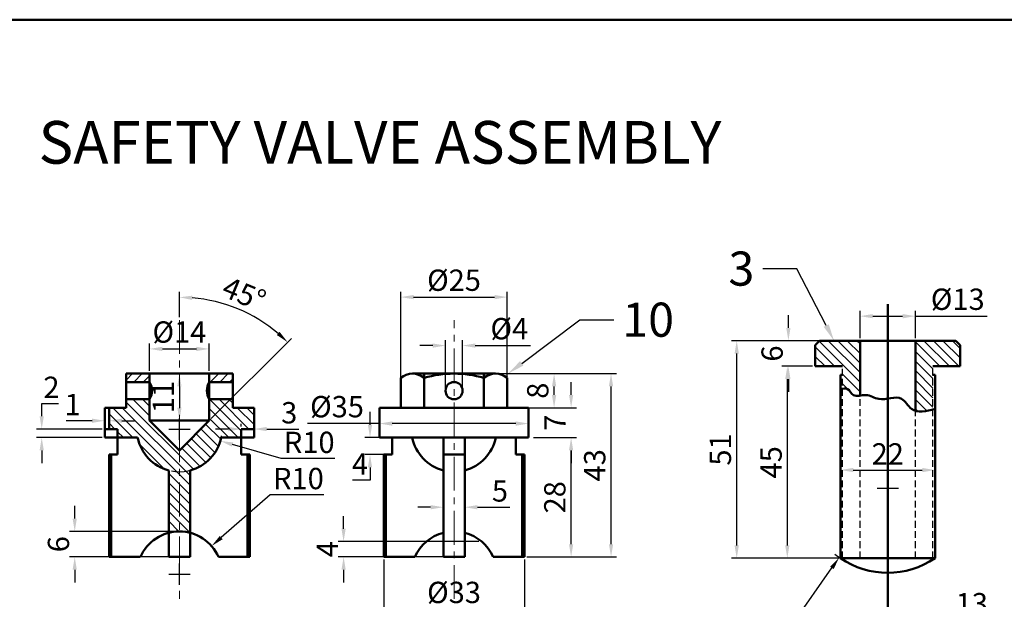
# Model space of a CAD drawing. Units: millimetres. Extents: x -656 to 85, y 134 to 571.
# Tile 4 of 5: x -409 to -178, y 435 to 571. Entities that reach past the tile are written whole.
import ezdxf
from ezdxf import colors
from ezdxf.entities.mleader import LeaderData, LeaderLine
from ezdxf.math import Vec2, Vec3

# ---------------------------------------------------------------- set-up
doc = ezdxf.new("R2010")
doc.units = ezdxf.units.MM
doc.header["$LTSCALE"] = 0.5
doc.linetypes.add('CENTER', pattern=[50.8, 31.75, -6.35, 6.35, -6.35])
doc.linetypes.add('HIDDEN', pattern=[9.525, 6.35, -3.175])
for name, color, linetype, lineweight in [('M-CNTR', 1, 'CENTER', 18), ('M-DIMS', 2, 'Continuous', 25), ('M-HATC', 8, 'Continuous', 18), ('M-HIDN', 3, 'HIDDEN', 25), ('M-OUTL', 7, 'Continuous', 50), ('M-TEXT', 7, 'Continuous', 25), ('M-TTLB', 7, 'Continuous', 50)]:
    doc.layers.add(name, color=color, linetype=linetype, lineweight=lineweight)
doc.styles.get("Standard").update_dxf_attribs({"font": 'arial.ttf'})
doc.dimstyles.new('ISO-25', dxfattribs={"dimtxt": 5, "dimasz": 3, "dimexe": 1.25, "dimexo": 0.625, "dimtad": 1, "dimtoh": 1, "dimdec": 0, "dimtxsty": 'Standard', "dimcen": 2.5, "dimadec": 0, "dimazin": 0, "dimtfac": 1, "dimtdec": 0, "dimtofl": 0, "dimtmove": 0, "dimatfit": 3, "dimfxl": 1, "dimarcsym": 0})

# ---------------------------------------------------------------- blocks, each defined once
blk = doc.blocks.new('*D33')
at = {"layer": 'Defpoints', "color": 0, "ltscale": 0.5, "transparency": 16777216}
for p in [(-323.49, 445.02), (-290.49, 445.02), (-290.49, 432.74)]:
    blk.add_point(p, dxfattribs=at)
at = {"layer": 'M-DIMS', "color": 0, "lineweight": -2, "ltscale": 0.5, "transparency": 16777216}
for p, q in [((-323.49, 444.4), (-323.49, 431.49)), ((-290.49, 444.4), (-290.49, 431.49)), ((-320.49, 432.74), (-293.49, 432.74))]:
    blk.add_line(p, q, dxfattribs=at)
at = {"layer": 'M-DIMS', "color": 0, "ltscale": 0.5, "transparency": 16777216}
for points in [[(-320.49, 433.24), (-320.49, 432.24), (-323.49, 432.74)], [(-293.49, 433.24), (-293.49, 432.24), (-290.49, 432.74)]]:
    blk.add_solid(points, dxfattribs=at)
at = {"layer": 'M-DIMS', "color": 0, "ltscale": 0.5, "transparency": 16777216, "insert": (-306.99, 436.06), "char_height": 5, "attachment_point": 5}
blk.add_mtext('%%C33', dxfattribs=at)
blk = doc.blocks.new('*D34')
at = {"layer": 'Defpoints', "color": 0, "ltscale": 0.5, "transparency": 16777216}
for p in [(-304.49, 456.69), (-309.49, 448.8), (-304.49, 448.8)]:
    blk.add_point(p, dxfattribs=at)
at = {"layer": 'M-DIMS', "color": 0, "lineweight": -2, "ltscale": 0.5, "transparency": 16777216}
for p, q in [((-309.49, 449.42), (-309.49, 457.94)), ((-304.49, 449.42), (-304.49, 457.94)), ((-312.49, 456.69), (-315.49, 456.69)), ((-301.49, 456.69), (-293.93, 456.69))]:
    blk.add_line(p, q, dxfattribs=at)
at = {"layer": 'M-DIMS', "color": 0, "ltscale": 0.5, "transparency": 16777216}
for points in [[(-312.49, 457.19), (-312.49, 456.19), (-309.49, 456.69)], [(-301.49, 457.19), (-301.49, 456.19), (-304.49, 456.69)]]:
    blk.add_solid(points, dxfattribs=at)
at = {"layer": 'M-DIMS', "color": 0, "ltscale": 0.5, "transparency": 16777216, "insert": (-296.21, 459.86), "char_height": 5, "attachment_point": 5}
blk.add_mtext('5', dxfattribs=at)
blk = doc.blocks.new('*D35')
at = {"layer": 'Defpoints', "color": 0, "ltscale": 0.5, "transparency": 16777216}
for p in [(-288.99, 473.02), (-279.52, 473.02), (-290.49, 445.02)]:
    blk.add_point(p, dxfattribs=at)
at = {"layer": 'M-DIMS', "color": 0, "lineweight": -2, "ltscale": 0.5, "transparency": 16777216}
for p, q in [((-288.37, 473.02), (-278.27, 473.02)), ((-279.52, 448.02), (-279.52, 470.02)), ((-289.87, 445.02), (-278.27, 445.02))]:
    blk.add_line(p, q, dxfattribs=at)
at = {"layer": 'M-DIMS', "color": 0, "ltscale": 0.5, "transparency": 16777216}
for points in [[(-280.02, 470.02), (-279.02, 470.02), (-279.52, 473.02)], [(-280.02, 448.02), (-279.02, 448.02), (-279.52, 445.02)]]:
    blk.add_solid(points, dxfattribs=at)
at = {"layer": 'M-DIMS', "color": 0, "ltscale": 0.5, "transparency": 16777216, "insert": (-282.69, 459.02), "char_height": 5, "attachment_point": 5, "rotation": 90}
blk.add_mtext('28', dxfattribs=at)
blk = doc.blocks.new('*D36')
at = {"layer": 'Defpoints', "color": 0, "ltscale": 0.5, "transparency": 16777216}
for p in [(-288.99, 480.02), (-279.52, 480.02), (-288.99, 473.02)]:
    blk.add_point(p, dxfattribs=at)
at = {"layer": 'M-DIMS', "color": 0, "lineweight": -2, "ltscale": 0.5, "transparency": 16777216}
for p, q in [((-279.52, 483.02), (-279.52, 486.02)), ((-288.37, 480.02), (-278.27, 480.02)), ((-288.37, 473.02), (-278.27, 473.02)), ((-279.52, 470.02), (-279.52, 467.02))]:
    blk.add_line(p, q, dxfattribs=at)
at = {"layer": 'M-DIMS', "color": 0, "ltscale": 0.5, "transparency": 16777216}
for points in [[(-280.02, 483.02), (-279.02, 483.02), (-279.52, 480.02)], [(-280.02, 470.02), (-279.02, 470.02), (-279.52, 473.02)]]:
    blk.add_solid(points, dxfattribs=at)
at = {"layer": 'M-DIMS', "color": 0, "ltscale": 0.5, "transparency": 16777216, "insert": (-282.64, 476.52), "char_height": 5, "attachment_point": 5, "rotation": 90}
blk.add_mtext('7', dxfattribs=at)
blk = doc.blocks.new('*D37')
at = {"layer": 'Defpoints', "color": 0, "ltscale": 0.5, "transparency": 16777216}
for p in [(-306.99, 488.02), (-270.15, 488.02), (-290.49, 445.02)]:
    blk.add_point(p, dxfattribs=at)
at = {"layer": 'M-DIMS', "color": 0, "lineweight": -2, "ltscale": 0.5, "transparency": 16777216}
for p, q in [((-306.37, 488.02), (-268.9, 488.02)), ((-270.15, 448.02), (-270.15, 485.02)), ((-289.87, 445.02), (-268.9, 445.02))]:
    blk.add_line(p, q, dxfattribs=at)
at = {"layer": 'M-DIMS', "color": 0, "ltscale": 0.5, "transparency": 16777216}
for points in [[(-270.65, 485.02), (-269.65, 485.02), (-270.15, 488.02)], [(-270.65, 448.02), (-269.65, 448.02), (-270.15, 445.02)]]:
    blk.add_solid(points, dxfattribs=at)
at = {"layer": 'M-DIMS', "color": 0, "ltscale": 0.5, "transparency": 16777216, "insert": (-273.33, 466.52), "char_height": 5, "attachment_point": 5, "rotation": 90}
blk.add_mtext('43', dxfattribs=at)
blk = doc.blocks.new('*D38')
at = {"layer": 'Defpoints', "color": 0, "ltscale": 0.5, "transparency": 16777216}
for p in [(-306.99, 488.02), (-283.51, 488.02), (-294.49, 480.02)]:
    blk.add_point(p, dxfattribs=at)
at = {"layer": 'M-DIMS', "color": 0, "lineweight": -2, "ltscale": 0.5, "transparency": 16777216}
for p, q in [((-306.37, 488.02), (-282.26, 488.02)), ((-283.51, 483.02), (-283.51, 485.02)), ((-293.87, 480.02), (-282.26, 480.02))]:
    blk.add_line(p, q, dxfattribs=at)
at = {"layer": 'M-DIMS', "color": 0, "ltscale": 0.5, "transparency": 16777216}
for points in [[(-284.01, 485.02), (-283.01, 485.02), (-283.51, 488.02)], [(-284.01, 483.02), (-283.01, 483.02), (-283.51, 480.02)]]:
    blk.add_solid(points, dxfattribs=at)
at = {"layer": 'M-DIMS', "color": 0, "ltscale": 0.5, "transparency": 16777216, "insert": (-286.69, 484.02), "char_height": 5, "attachment_point": 5, "rotation": 90}
blk.add_mtext('8', dxfattribs=at)
blk = doc.blocks.new('*D39')
at = {"layer": 'Defpoints', "color": 0, "ltscale": 0.5, "transparency": 16777216}
for p in [(-294.49, 505.96), (-319.49, 483.52), (-294.49, 483.52)]:
    blk.add_point(p, dxfattribs=at)
at = {"layer": 'M-DIMS', "color": 0, "lineweight": -2, "ltscale": 0.5, "transparency": 16777216}
for p, q in [((-319.49, 484.15), (-319.49, 507.21)), ((-316.49, 505.96), (-297.49, 505.96)), ((-294.49, 484.15), (-294.49, 507.21))]:
    blk.add_line(p, q, dxfattribs=at)
at = {"layer": 'M-DIMS', "color": 0, "ltscale": 0.5, "transparency": 16777216}
for points in [[(-316.49, 506.46), (-316.49, 505.46), (-319.49, 505.96)], [(-297.49, 506.46), (-297.49, 505.46), (-294.49, 505.96)]]:
    blk.add_solid(points, dxfattribs=at)
at = {"layer": 'M-DIMS', "color": 0, "ltscale": 0.5, "transparency": 16777216, "insert": (-306.99, 509.28), "char_height": 5, "attachment_point": 5}
blk.add_mtext('%%C25', dxfattribs=at)
blk = doc.blocks.new('*D40')
at = {"layer": 'Defpoints', "color": 0, "ltscale": 0.5, "transparency": 16777216}
for p in [(-304.99, 494.59), (-308.99, 484.02), (-304.99, 484.02)]:
    blk.add_point(p, dxfattribs=at)
at = {"layer": 'M-DIMS', "color": 0, "lineweight": -2, "ltscale": 0.5, "transparency": 16777216}
for p, q in [((-311.99, 494.59), (-314.99, 494.59)), ((-308.99, 484.65), (-308.99, 495.84)), ((-304.99, 484.65), (-304.99, 495.84)), ((-301.99, 494.59), (-289.04, 494.59))]:
    blk.add_line(p, q, dxfattribs=at)
at = {"layer": 'M-DIMS', "color": 0, "ltscale": 0.5, "transparency": 16777216}
for points in [[(-311.99, 495.09), (-311.99, 494.09), (-308.99, 494.59)], [(-301.99, 495.09), (-301.99, 494.09), (-304.99, 494.59)]]:
    blk.add_solid(points, dxfattribs=at)
at = {"layer": 'M-DIMS', "color": 0, "ltscale": 0.5, "transparency": 16777216, "insert": (-294.02, 497.91), "char_height": 5, "attachment_point": 5}
blk.add_mtext('%%C4', dxfattribs=at)
blk = doc.blocks.new('*D41')
at = {"layer": 'Defpoints', "color": 0, "ltscale": 0.5, "transparency": 16777216}
for p in [(-324.49, 476.52), (-289.49, 476.52), (-289.49, 476.31)]:
    blk.add_point(p, dxfattribs=at)
at = {"layer": 'M-DIMS', "color": 0, "lineweight": -2, "ltscale": 0.5, "transparency": 16777216}
for p, q in [((-324.49, 476.31), (-341.38, 476.31)), ((-292.49, 476.31), (-321.49, 476.31)), ((-324.49, 475.9), (-324.49, 475.06)), ((-289.49, 475.9), (-289.49, 475.06))]:
    blk.add_line(p, q, dxfattribs=at)
at = {"layer": 'M-DIMS', "color": 0, "ltscale": 0.5, "transparency": 16777216}
for points in [[(-321.49, 476.81), (-321.49, 475.81), (-324.49, 476.31)], [(-292.49, 476.81), (-292.49, 475.81), (-289.49, 476.31)]]:
    blk.add_solid(points, dxfattribs=at)
at = {"layer": 'M-DIMS', "color": 0, "ltscale": 0.5, "transparency": 16777216, "insert": (-334.44, 479.62), "char_height": 5, "attachment_point": 5}
blk.add_mtext('%%C35', dxfattribs=at)
blk = doc.blocks.new('*D42')
at = {"layer": 'Defpoints', "color": 0, "ltscale": 0.5, "transparency": 16777216}
for p in [(-321.49, 473.02), (-326.7, 469.02), (-321.49, 469.02)]:
    blk.add_point(p, dxfattribs=at)
at = {"layer": 'M-DIMS', "color": 0, "lineweight": -2, "ltscale": 0.5, "transparency": 16777216}
for p, q in [((-326.7, 476.02), (-326.7, 479.02)), ((-322.12, 473.02), (-327.95, 473.02)), ((-322.12, 469.02), (-327.95, 469.02)), ((-326.7, 466.02), (-326.7, 463.02)), ((-326.7, 463.02), (-330.78, 463.02))]:
    blk.add_line(p, q, dxfattribs=at)
at = {"layer": 'M-DIMS', "color": 0, "ltscale": 0.5, "transparency": 16777216}
for points in [[(-327.2, 476.02), (-326.2, 476.02), (-326.7, 473.02)], [(-327.2, 466.02), (-326.2, 466.02), (-326.7, 469.02)]]:
    blk.add_solid(points, dxfattribs=at)
at = {"layer": 'M-DIMS', "color": 0, "ltscale": 0.5, "transparency": 16777216, "insert": (-329.05, 466.15), "char_height": 5, "attachment_point": 5}
blk.add_mtext('4', dxfattribs=at)
blk = doc.blocks.new('*D43')
at = {"layer": 'Defpoints', "color": 0, "ltscale": 0.5, "transparency": 16777216}
for p in [(-364.42, 493.81), (-378.42, 488.02), (-364.42, 488.02)]:
    blk.add_point(p, dxfattribs=at)
at = {"layer": 'M-DIMS', "color": 0, "lineweight": -2, "ltscale": 0.5, "transparency": 16777216}
for p, q in [((-378.42, 488.65), (-378.42, 495.06)), ((-364.42, 488.65), (-364.42, 495.06)), ((-375.42, 493.81), (-367.42, 493.81))]:
    blk.add_line(p, q, dxfattribs=at)
at = {"layer": 'M-DIMS', "color": 0, "ltscale": 0.5, "transparency": 16777216}
for points in [[(-375.42, 494.31), (-375.42, 493.31), (-378.42, 493.81)], [(-367.42, 494.31), (-367.42, 493.31), (-364.42, 493.81)]]:
    blk.add_solid(points, dxfattribs=at)
at = {"layer": 'M-DIMS', "color": 0, "ltscale": 0.5, "transparency": 16777216, "insert": (-371.42, 497.12), "char_height": 5, "attachment_point": 5}
blk.add_mtext('%%C14', dxfattribs=at)
blk = doc.blocks.new('*D44')
at = {"layer": 'Defpoints', "color": 0, "ltscale": 0.5, "transparency": 16777216}
for p in [(-403.73, 475.02), (-388.92, 475.02), (-388.92, 473.02)]:
    blk.add_point(p, dxfattribs=at)
at = {"layer": 'M-DIMS', "color": 0, "lineweight": -2, "ltscale": 0.5, "transparency": 16777216}
for p, q in [((-403.73, 478.02), (-403.73, 481.02)), ((-403.73, 481.02), (-399.79, 481.02)), ((-389.55, 475.02), (-404.98, 475.02)), ((-389.55, 473.02), (-404.98, 473.02)), ((-403.73, 470.02), (-403.73, 467.02))]:
    blk.add_line(p, q, dxfattribs=at)
at = {"layer": 'M-DIMS', "color": 0, "ltscale": 0.5, "transparency": 16777216}
for points in [[(-404.23, 478.02), (-403.23, 478.02), (-403.73, 475.02)], [(-404.23, 470.02), (-403.23, 470.02), (-403.73, 473.02)]]:
    blk.add_solid(points, dxfattribs=at)
at = {"layer": 'M-DIMS', "color": 0, "ltscale": 0.5, "transparency": 16777216, "insert": (-401.44, 484.16), "char_height": 5, "attachment_point": 5}
blk.add_mtext('2', dxfattribs=at)
blk = doc.blocks.new('*D45')
at = {"layer": 'Defpoints', "color": 0, "ltscale": 0.5, "transparency": 16777216}
for p in [(-388.92, 476.52), (-387.92, 476.97), (-387.92, 476.52)]:
    blk.add_point(p, dxfattribs=at)
at = {"layer": 'M-DIMS', "color": 0, "lineweight": -2, "ltscale": 0.5, "transparency": 16777216}
for p, q in [((-388.92, 477.15), (-388.92, 478.22)), ((-387.92, 477.15), (-387.92, 478.22)), ((-391.92, 476.97), (-398.01, 476.97)), ((-384.92, 476.97), (-381.92, 476.97))]:
    blk.add_line(p, q, dxfattribs=at)
at = {"layer": 'M-DIMS', "color": 0, "ltscale": 0.5, "transparency": 16777216}
for points in [[(-391.92, 477.47), (-391.92, 476.47), (-388.92, 476.97)], [(-384.92, 477.47), (-384.92, 476.47), (-387.92, 476.97)]]:
    blk.add_solid(points, dxfattribs=at)
at = {"layer": 'M-DIMS', "color": 0, "ltscale": 0.5, "transparency": 16777216, "insert": (-396.47, 480.11), "char_height": 5, "attachment_point": 5}
blk.add_mtext('1', dxfattribs=at)
blk = doc.blocks.new('*D46')
at = {"layer": 'Defpoints', "color": 0, "ltscale": 0.5, "transparency": 16777216}
for p in [(-356.92, 475.02), (-353.92, 475.02), (-353.92, 475.02)]:
    blk.add_point(p, dxfattribs=at)
at = {"layer": 'M-DIMS', "color": 0, "lineweight": -2, "ltscale": 0.5, "transparency": 16777216}
for p, q in [((-356.92, 475.65), (-356.92, 476.27)), ((-353.92, 475.65), (-353.92, 476.27)), ((-359.92, 475.02), (-362.92, 475.02)), ((-350.92, 475.02), (-343.4, 475.02))]:
    blk.add_line(p, q, dxfattribs=at)
at = {"layer": 'M-DIMS', "color": 0, "ltscale": 0.5, "transparency": 16777216}
for points in [[(-359.92, 475.52), (-359.92, 474.52), (-356.92, 475.02)], [(-350.92, 475.52), (-350.92, 474.52), (-353.92, 475.02)]]:
    blk.add_solid(points, dxfattribs=at)
at = {"layer": 'M-DIMS', "color": 0, "ltscale": 0.5, "transparency": 16777216, "insert": (-345.66, 478.2), "char_height": 5, "attachment_point": 5}
blk.add_mtext('3', dxfattribs=at)
blk = doc.blocks.new('*D47')
at = {"layer": 'Defpoints', "color": 0, "ltscale": 0.5, "transparency": 16777216}
for p in [(-371.42, 475.02), (-361.82, 472.23)]:
    blk.add_point(p, dxfattribs=at)
at = {"layer": 'M-DIMS', "color": 0, "lineweight": -2, "ltscale": 0.5, "transparency": 16777216}
for p, q in [((-371.42, 472.52), (-371.42, 477.52)), ((-373.92, 475.02), (-368.92, 475.02)), ((-347.55, 468.08), (-358.94, 471.39)), ((-334.99, 468.08), (-347.55, 468.08))]:
    blk.add_line(p, q, dxfattribs=at)
blk.add_arc((-371.42, 475.02), 10, 259.1035, 350.9346, dxfattribs=at)
at = {"layer": 'M-DIMS', "color": 0, "ltscale": 0.5, "transparency": 16777216}
blk.add_solid([(-358.8, 471.87), (-359.08, 470.91), (-361.82, 472.23)], dxfattribs=at)
at = {"layer": 'M-DIMS', "color": 0, "ltscale": 0.5, "transparency": 16777216, "insert": (-340.96, 471.25), "char_height": 5, "attachment_point": 5}
blk.add_mtext('R10', dxfattribs=at)
blk = doc.blocks.new('*D48')
at = {"layer": 'Defpoints', "color": 0, "ltscale": 0.5, "transparency": 16777216}
for p in [(-371.42, 500.59), (-353.47, 501.11), (-364.42, 477.02), (-371.42, 470.02), (-371.42, 435.19)]:
    blk.add_point(p, dxfattribs=at)
at = {"layer": 'M-DIMS', "color": 0, "lineweight": -2, "ltscale": 0.5, "transparency": 16777216}
for p, q in [((-371.42, 501.22), (-371.42, 507.17)), ((-363.98, 477.47), (-345.15, 496.29))]:
    blk.add_line(p, q, dxfattribs=at)
blk.add_arc((-371.42, 470.02), 35.9, 49.7896, 85.2104, dxfattribs=at)
at = {"layer": 'M-DIMS', "color": 0, "ltscale": 0.5, "transparency": 16777216}
for points in [[(-368.45, 505.3), (-368.4, 506.3), (-371.42, 505.92)], [(-347.91, 497.81), (-348.58, 497.07), (-346.04, 495.41)]]:
    blk.add_solid(points, dxfattribs=at)
at = {"layer": 'M-DIMS', "color": 0, "ltscale": 0.5, "transparency": 16777216, "insert": (-356.47, 506.12), "char_height": 5, "attachment_point": 5, "rotation": 337.5}
blk.add_mtext('45°', dxfattribs=at)
blk = doc.blocks.new('*D49')
at = {"layer": 'Defpoints', "color": 0, "ltscale": 0.5, "transparency": 16777216}
for p in [(-372.99, 488.02), (-372.99, 477.02), (-371.42, 477.02)]:
    blk.add_point(p, dxfattribs=at)
at = {"layer": 'M-DIMS', "color": 0, "lineweight": -2, "ltscale": 0.5, "transparency": 16777216}
for p, q in [((-372.36, 488.02), (-370.17, 488.02)), ((-371.42, 485.02), (-371.42, 480.02)), ((-372.36, 477.02), (-370.17, 477.02))]:
    blk.add_line(p, q, dxfattribs=at)
at = {"layer": 'M-DIMS', "color": 0, "ltscale": 0.5, "transparency": 16777216}
for points in [[(-371.92, 485.02), (-370.92, 485.02), (-371.42, 488.02)], [(-371.92, 480.02), (-370.92, 480.02), (-371.42, 477.02)]]:
    blk.add_solid(points, dxfattribs=at)
at = {"layer": 'M-DIMS', "color": 0, "ltscale": 0.5, "transparency": 16777216, "insert": (-374.56, 482.52), "char_height": 5, "attachment_point": 5, "rotation": 90}
blk.add_mtext('11', dxfattribs=at)
blk = doc.blocks.new('*D51')
at = {"layer": 'Defpoints', "color": 0, "ltscale": 0.5, "transparency": 16777216}
for p in [(-200.1, 422), (-200.08, 421.98), (-210.36, 414.02)]:
    blk.add_point(p, dxfattribs=at)
at = {"layer": 'M-DIMS', "color": 0, "lineweight": -2, "ltscale": 0.5, "transparency": 16777216}
for p, q in [((-200.08, 421.98), (-189.47, 430.24)), ((-189.47, 430.24), (-182.15, 430.24)), ((-199.72, 421.51), (-199.32, 420.99)), ((-207.97, 415.83), (-202.45, 420.13)), ((-209.98, 413.52), (-209.57, 413.01))]:
    blk.add_line(p, q, dxfattribs=at)
at = {"layer": 'M-DIMS', "color": 0, "ltscale": 0.5, "transparency": 16777216}
for points in [[(-202.76, 420.53), (-202.14, 419.74), (-200.08, 421.98)], [(-208.28, 416.23), (-207.67, 415.44), (-210.34, 413.99)]]:
    blk.add_solid(points, dxfattribs=at)
at = {"layer": 'M-DIMS', "color": 0, "ltscale": 0.5, "transparency": 16777216, "insert": (-185.5, 433.42), "char_height": 5, "attachment_point": 5}
blk.add_mtext('13', dxfattribs=at)
blk = doc.blocks.new('*D52')
at = {"layer": 'Defpoints', "color": 0, "ltscale": 0.5, "transparency": 16777216}
for p in [(-228.54, 495.73), (-205.23, 495.73), (-222.23, 489.73)]:
    blk.add_point(p, dxfattribs=at)
at = {"layer": 'M-DIMS', "color": 0, "lineweight": -2, "ltscale": 0.5, "transparency": 16777216}
for p, q in [((-228.54, 498.73), (-228.54, 501.73)), ((-205.86, 495.73), (-229.79, 495.73)), ((-222.86, 489.73), (-229.79, 489.73)), ((-228.54, 486.73), (-228.54, 483.73))]:
    blk.add_line(p, q, dxfattribs=at)
at = {"layer": 'M-DIMS', "color": 0, "ltscale": 0.5, "transparency": 16777216}
for points in [[(-229.04, 498.73), (-228.04, 498.73), (-228.54, 495.73)], [(-229.04, 486.73), (-228.04, 486.73), (-228.54, 489.73)]]:
    blk.add_solid(points, dxfattribs=at)
at = {"layer": 'M-DIMS', "color": 0, "ltscale": 0.5, "transparency": 16777216, "insert": (-231.71, 492.73), "char_height": 5, "attachment_point": 5, "rotation": 90}
blk.add_mtext('6', dxfattribs=at)
blk = doc.blocks.new('*D53')
at = {"layer": 'Defpoints', "color": 0, "ltscale": 0.5, "transparency": 16777216}
for p in [(-240.66, 495.73), (-205.23, 495.73), (-205.23, 444.73)]:
    blk.add_point(p, dxfattribs=at)
at = {"layer": 'M-DIMS', "color": 0, "lineweight": -2, "ltscale": 0.5, "transparency": 16777216}
for p, q in [((-205.86, 495.73), (-241.91, 495.73)), ((-240.66, 447.73), (-240.66, 492.73)), ((-205.86, 444.73), (-241.91, 444.73))]:
    blk.add_line(p, q, dxfattribs=at)
at = {"layer": 'M-DIMS', "color": 0, "ltscale": 0.5, "transparency": 16777216}
for points in [[(-241.16, 492.73), (-240.16, 492.73), (-240.66, 495.73)], [(-241.16, 447.73), (-240.16, 447.73), (-240.66, 444.73)]]:
    blk.add_solid(points, dxfattribs=at)
at = {"layer": 'M-DIMS', "color": 0, "ltscale": 0.5, "transparency": 16777216, "insert": (-243.84, 470.23), "char_height": 5, "attachment_point": 5, "rotation": 90}
blk.add_mtext('51', dxfattribs=at)
blk = doc.blocks.new('*D54')
at = {"layer": 'Defpoints', "color": 0, "ltscale": 0.5, "transparency": 16777216}
for p in [(-205.23, 461.18), (-216.61, 444.92)]:
    blk.add_point(p, dxfattribs=at)
at = {"layer": 'M-DIMS', "color": 0, "lineweight": -2, "ltscale": 0.5, "transparency": 16777216}
for p, q in [((-205.23, 458.68), (-205.23, 463.68)), ((-207.73, 461.18), (-202.73, 461.18)), ((-232.53, 422.16), (-218.33, 442.46)), ((-249.97, 422.16), (-232.53, 422.16))]:
    blk.add_line(p, q, dxfattribs=at)
blk.add_arc((-205.23, 461.18), 19.85, 231.4164, 235.9903, dxfattribs=at)
at = {"layer": 'M-DIMS', "color": 0, "ltscale": 0.5, "transparency": 16777216}
blk.add_solid([(-218.74, 442.75), (-217.92, 442.18), (-216.61, 444.92)], dxfattribs=at)
at = {"layer": 'M-DIMS', "color": 0, "ltscale": 0.5, "transparency": 16777216, "insert": (-244, 425.34), "char_height": 5, "attachment_point": 5}
blk.add_mtext('R20', dxfattribs=at)
blk = doc.blocks.new('*D55')
at = {"layer": 'Defpoints', "color": 0, "ltscale": 0.5, "transparency": 16777216}
for p in [(-216.33, 466.23), (-194.13, 466.23), (-194.13, 465.41)]:
    blk.add_point(p, dxfattribs=at)
at = {"layer": 'M-DIMS', "color": 0, "lineweight": -2, "ltscale": 0.5, "transparency": 16777216}
for p, q in [((-216.33, 465.61), (-216.33, 464.16)), ((-213.33, 465.41), (-197.13, 465.41)), ((-194.13, 465.61), (-194.13, 464.16))]:
    blk.add_line(p, q, dxfattribs=at)
at = {"layer": 'M-DIMS', "color": 0, "ltscale": 0.5, "transparency": 16777216}
for points in [[(-213.33, 465.91), (-213.33, 464.91), (-216.33, 465.41)], [(-197.13, 465.91), (-197.13, 464.91), (-194.13, 465.41)]]:
    blk.add_solid(points, dxfattribs=at)
at = {"layer": 'M-DIMS', "color": 0, "ltscale": 0.5, "transparency": 16777216, "insert": (-205.23, 468.54), "char_height": 5, "attachment_point": 5}
blk.add_mtext('22', dxfattribs=at)
blk = doc.blocks.new('*D71')
at = {"layer": 'Defpoints', "color": 0, "ltscale": 0.5, "transparency": 16777216}
for p in [(-222.23, 489.73), (-228.79, 444.73), (-223.88, 444.73)]:
    blk.add_point(p, dxfattribs=at)
at = {"layer": 'M-DIMS', "color": 0, "lineweight": -2, "ltscale": 0.5, "transparency": 16777216}
for p, q in [((-222.86, 489.73), (-230.04, 489.73)), ((-228.79, 486.73), (-228.79, 447.73)), ((-224.51, 444.73), (-230.04, 444.73))]:
    blk.add_line(p, q, dxfattribs=at)
at = {"layer": 'M-DIMS', "color": 0, "ltscale": 0.5, "transparency": 16777216}
for points in [[(-229.29, 486.73), (-228.29, 486.73), (-228.79, 489.73)], [(-229.29, 447.73), (-228.29, 447.73), (-228.79, 444.73)]]:
    blk.add_solid(points, dxfattribs=at)
at = {"layer": 'M-DIMS', "color": 0, "ltscale": 0.5, "transparency": 16777216, "insert": (-231.95, 467.23), "char_height": 5, "attachment_point": 5, "rotation": 90}
blk.add_mtext('45', dxfattribs=at)
blk = doc.blocks.new('*D78')
at = {"layer": 'Defpoints', "color": 0, "ltscale": 0.5, "transparency": 16777216}
for p in [(-198.73, 501.49), (-211.73, 495.73), (-198.73, 495.73)]:
    blk.add_point(p, dxfattribs=at)
at = {"layer": 'M-DIMS', "color": 0, "lineweight": -2, "ltscale": 0.5, "transparency": 16777216}
for p, q in [((-211.73, 496.36), (-211.73, 502.74)), ((-208.73, 501.49), (-201.73, 501.49)), ((-198.73, 496.36), (-198.73, 502.74)), ((-198.73, 501.49), (-181.88, 501.49))]:
    blk.add_line(p, q, dxfattribs=at)
at = {"layer": 'M-DIMS', "color": 0, "ltscale": 0.5, "transparency": 16777216}
for points in [[(-208.73, 501.99), (-208.73, 500.99), (-211.73, 501.49)], [(-201.73, 501.99), (-201.73, 500.99), (-198.73, 501.49)]]:
    blk.add_solid(points, dxfattribs=at)
at = {"layer": 'M-DIMS', "color": 0, "ltscale": 0.5, "transparency": 16777216, "insert": (-188.8, 504.81), "char_height": 5, "attachment_point": 5}
blk.add_mtext('%%C13', dxfattribs=at)
blk = doc.blocks.new('*D79')
at = {"layer": 'Defpoints', "color": 0, "ltscale": 0.5, "transparency": 16777216}
for p in [(-300.5, 448.63), (-332.9, 445.02), (-306.99, 445.02)]:
    blk.add_point(p, dxfattribs=at)
at = {"layer": 'M-DIMS', "color": 0, "lineweight": -2, "ltscale": 0.5, "transparency": 16777216}
for p, q in [((-332.9, 451.63), (-332.9, 454.63)), ((-301.13, 448.63), (-334.15, 448.63)), ((-307.62, 445.02), (-334.15, 445.02)), ((-332.9, 442.02), (-332.9, 439.02))]:
    blk.add_line(p, q, dxfattribs=at)
at = {"layer": 'M-DIMS', "color": 0, "ltscale": 0.5, "transparency": 16777216}
for points in [[(-333.4, 451.63), (-332.4, 451.63), (-332.9, 448.63)], [(-333.4, 442.02), (-332.4, 442.02), (-332.9, 445.02)]]:
    blk.add_solid(points, dxfattribs=at)
at = {"layer": 'M-DIMS', "color": 0, "ltscale": 0.5, "transparency": 16777216, "insert": (-336.03, 446.83), "char_height": 5, "attachment_point": 5, "rotation": 90}
blk.add_mtext('4', dxfattribs=at)
blk = doc.blocks.new('*D80')
at = {"layer": 'Defpoints', "color": 0, "ltscale": 0.5, "transparency": 16777216}
for p in [(-371.42, 451.02), (-395.98, 445.02), (-371.42, 445.02)]:
    blk.add_point(p, dxfattribs=at)
at = {"layer": 'M-DIMS', "color": 0, "lineweight": -2, "ltscale": 0.5, "transparency": 16777216}
for p, q in [((-395.98, 454.02), (-395.98, 457.02)), ((-372.05, 451.02), (-397.23, 451.02)), ((-372.05, 445.02), (-397.23, 445.02)), ((-395.98, 442.02), (-395.98, 439.02))]:
    blk.add_line(p, q, dxfattribs=at)
at = {"layer": 'M-DIMS', "color": 0, "ltscale": 0.5, "transparency": 16777216}
for points in [[(-396.48, 454.02), (-395.48, 454.02), (-395.98, 451.02)], [(-396.48, 442.02), (-395.48, 442.02), (-395.98, 445.02)]]:
    blk.add_solid(points, dxfattribs=at)
at = {"layer": 'M-DIMS', "color": 0, "ltscale": 0.5, "transparency": 16777216, "insert": (-399.15, 448.02), "char_height": 5, "attachment_point": 5, "rotation": 90}
blk.add_mtext('6', dxfattribs=at)
blk = doc.blocks.new('*D81')
at = {"layer": 'Defpoints', "color": 0, "ltscale": 0.5, "transparency": 16777216}
for p in [(-363.88, 447.59), (-371.42, 441.02)]:
    blk.add_point(p, dxfattribs=at)
at = {"layer": 'M-DIMS', "color": 0, "lineweight": -2, "ltscale": 0.5, "transparency": 16777216}
for p, q in [((-350.09, 459.59), (-361.62, 449.56)), ((-337.53, 459.59), (-350.09, 459.59)), ((-371.42, 438.52), (-371.42, 443.52)), ((-373.92, 441.02), (-368.92, 441.02))]:
    blk.add_line(p, q, dxfattribs=at)
at = {"layer": 'M-DIMS', "color": 0, "ltscale": 0.5, "transparency": 16777216}
blk.add_solid([(-361.95, 449.94), (-361.29, 449.18), (-363.88, 447.59)], dxfattribs=at)
at = {"layer": 'M-DIMS', "color": 0, "ltscale": 0.5, "transparency": 16777216, "insert": (-343.5, 462.77), "char_height": 5, "attachment_point": 5}
blk.add_mtext('R10', dxfattribs=at)

msp = doc.modelspace()

# ---------------------------------------------------------------- hatches: boundary and pattern name
at = {"layer": 'M-HATC', "ltscale": 0.5}
h = msp.add_hatch(dxfattribs=at)
h.set_pattern_fill('ANSI31', color=256, scale=0.5, angle=90)
h.set_pattern_definition([(135, (-1699.1516, -78.561), (-1.122532, -1.122532), [])])
edge = h.paths.add_edge_path()
edge.add_line((-211.73, 495.73), (-221.23, 495.73))
edge.add_line((-221.23, 495.73), (-222.23, 494.73))
edge.add_line((-222.23, 494.73), (-222.23, 489.73))
edge.add_line((-222.23, 489.73), (-215.83, 489.73))
edge.add_line((-215.83, 489.73), (-215.83, 484.49))
edge.add_spline(control_points=[(-215.83, 484.49), (-215.41, 484.55), (-214.33, 484.59), (-213.51, 482.67), (-212.3, 482.76), (-211.73, 482.84)], knot_values=[0.462825, 0.462825, 0.462825, 0.462825, 1.655207, 3.649135, 5.265139, 5.265139, 5.265139, 5.265139], degree=3, periodic=0)
edge.add_line((-211.73, 482.84), (-211.73, 495.73))
h.paths.add_polyline_path([(-188.23, 494.73), (-189.23, 495.73), (-198.73, 495.73), (-198.73, 489.73), (-188.23, 489.73)])
edge = h.paths.add_edge_path()
edge.add_line((-194.63, 489.73), (-198.73, 489.73))
edge.add_line((-198.73, 489.73), (-198.73, 479.3))
edge.add_spline(control_points=[(-198.73, 479.3), (-197.55, 478.95), (-196.11, 479.26), (-194.63, 479.63)], knot_values=[19.465698, 19.465698, 19.465698, 19.465698, 23.432296, 23.432296, 23.432296, 23.432296], degree=3, periodic=0)
edge.add_line((-194.63, 479.63), (-194.63, 489.73))
h = msp.add_hatch(dxfattribs=at)
h.set_pattern_fill('ANSI31', color=256, scale=0.5)
h.set_pattern_definition([(45, (-1712.0703, 33.9183), (-1.122532, 1.122532), [])])
h.paths.add_polyline_path([(-358.92, 488.02), (-364.42, 488.02), (-364.42, 486.02), (-358.92, 486.02)])
h.paths.add_polyline_path([(-378.42, 488.02), (-383.92, 488.02), (-383.92, 486.02), (-378.42, 486.02)])
edge = h.paths.add_edge_path()
edge.add_arc((-371.42, 441.02), 10, 90, 104.4775)
edge.add_line((-373.92, 450.71), (-373.92, 450.35))
edge.add_arc((-371.42, 446.02), 5, 90, 120, ccw=False)
h = msp.add_hatch(dxfattribs=at)
h.set_pattern_fill('ANSI31', color=256, scale=0.5, angle=90)
h.set_pattern_definition([(135, (-1507.2803, -236.2308), (-1.122532, -1.122532), [])])
h.paths.add_polyline_path([(-373.92, 465.34), (-373.92, 450.71, -0.063254), (-371.42, 451.02), (-371.42, 470.02), (-378.42, 477.02), (-378.42, 482.02), (-383.92, 482.02), (-383.92, 480.02), (-387.92, 480.02), (-387.92, 475.02), (-385.92, 475.02), (-385.92, 473.02), (-381.22, 473.02, 0.286677)])
h.paths.add_polyline_path([(-361.62, 473.02), (-356.92, 473.02), (-356.92, 475.02), (-353.92, 475.02), (-353.92, 480.02), (-358.92, 480.02), (-358.92, 482.02), (-364.42, 482.02), (-364.42, 477.02), (-371.42, 470.02), (-371.42, 451.02, -0.063254), (-368.92, 450.71), (-368.92, 465.34, 0.286677)])

# ---------------------------------------------------------------- linework, layer by layer
at = {"layer": 'M-CNTR', "ltscale": 0.5}
for p, q in [((-371.42, 500.59), (-371.42, 435.19)), ((-306.99, 435.19), (-306.99, 500.59))]:
    msp.add_line(p, q, dxfattribs=at)
at = {"layer": 'M-HIDN', "ltscale": 0.5}
for p, q in [((-215.83, 444.73), (-215.83, 489.73)), ((-194.63, 444.73), (-194.63, 489.73)), ((-211.73, 444.73), (-211.73, 482.84)), ((-198.73, 444.73), (-198.73, 479.3))]:
    msp.add_line(p, q, dxfattribs=at)
at = {"layer": 'M-OUTL', "ltscale": 0.5}
for p, q in [((-205.23, 394.53), (-205.23, 504.27)), ((-222.23, 494.73), (-221.23, 495.73)), ((-222.23, 489.73), (-222.23, 494.73)), ((-221.23, 495.73), (-189.23, 495.73)), ((-211.73, 482.84), (-211.73, 495.73)), ((-198.73, 479.3), (-198.73, 495.73)), ((-189.23, 495.73), (-188.23, 494.73)), ((-188.23, 494.73), (-188.23, 489.73)), ((-383.92, 480.02), (-383.92, 488.02)), ((-383.92, 488.02), (-358.92, 488.02)), ((-378.42, 477.02), (-378.42, 488.02)), ((-364.42, 488.02), (-364.42, 477.02)), ((-358.92, 488.02), (-358.92, 480.02)), ((-316.74, 488.02), (-297.24, 488.02)), ((-313.99, 480.02), (-313.99, 488.02)), ((-299.99, 488.02), (-299.99, 480.02)), ((-215.83, 489.73), (-222.23, 489.73)), ((-216.33, 444.73), (-216.33, 487.73)), ((-215.83, 487.73), (-216.33, 487.73)), ((-188.23, 489.73), (-194.63, 489.73)), ((-194.13, 487.73), (-194.63, 487.73)), ((-194.13, 444.73), (-194.13, 487.73)), ((-383.92, 486.02), (-378.42, 486.02)), ((-364.42, 486.02), (-358.92, 486.02)), ((-319.49, 480.02), (-319.49, 487.02)), ((-294.49, 487.02), (-294.49, 480.02)), ((-383.92, 482.02), (-378.42, 482.02)), ((-364.42, 482.02), (-358.92, 482.02)), ((-388.92, 473.02), (-388.92, 480.02)), ((-388.92, 480.02), (-383.92, 480.02)), ((-387.92, 475.02), (-387.92, 480.02)), ((-358.92, 480.02), (-353.92, 480.02)), ((-353.92, 480.02), (-353.92, 473.02)), ((-324.49, 473.02), (-324.49, 480.02)), ((-324.49, 480.02), (-289.49, 480.02)), ((-289.49, 480.02), (-289.49, 473.02)), ((-364.42, 477.02), (-378.42, 477.02)), ((-378.42, 477.02), (-371.42, 470.02)), ((-364.42, 477.02), (-371.42, 470.02)), ((-385.92, 475.02), (-388.92, 475.02)), ((-385.92, 475.02), (-385.92, 469.02)), ((-356.92, 475.02), (-356.92, 469.02)), ((-353.92, 475.02), (-356.92, 475.02)), ((-381.22, 473.02), (-388.92, 473.02)), ((-353.92, 473.02), (-361.62, 473.02)), ((-289.49, 473.02), (-324.49, 473.02)), ((-321.49, 473.02), (-321.49, 469.02)), ((-309.49, 473.02), (-309.49, 445.02)), ((-304.49, 473.02), (-304.49, 445.02)), ((-292.49, 473.02), (-292.49, 469.02)), ((-387.92, 469.02), (-387.92, 445.02)), ((-385.92, 469.02), (-387.92, 469.02)), ((-387.42, 469.02), (-387.42, 445.02)), ((-356.92, 469.02), (-354.92, 469.02)), ((-355.42, 469.02), (-355.42, 445.02)), ((-354.92, 469.02), (-354.92, 445.02)), ((-323.49, 469.02), (-323.49, 445.02)), ((-321.49, 469.02), (-323.49, 469.02)), ((-322.99, 469.02), (-322.99, 445.02)), ((-309.49, 469.02), (-304.49, 469.02)), ((-292.49, 469.02), (-290.49, 469.02)), ((-290.99, 469.02), (-290.99, 445.02)), ((-290.49, 469.02), (-290.49, 445.02)), ((-373.92, 465.34), (-373.92, 445.02)), ((-368.92, 465.34), (-368.92, 445.02)), ((-387.92, 445.02), (-380.59, 445.02)), ((-373.92, 445.02), (-368.92, 445.02)), ((-373.92, 445.02), (-368.92, 445.02)), ((-362.26, 445.02), (-354.92, 445.02)), ((-323.49, 445.02), (-322.99, 445.02)), ((-323.49, 445.02), (-316.16, 445.02)), ((-309.49, 445.02), (-304.49, 445.02)), ((-309.49, 445.02), (-304.49, 445.02)), ((-297.83, 445.02), (-290.49, 445.02)), ((-216.33, 444.73), (-194.13, 444.73))]:
    msp.add_line(p, q, dxfattribs=at)
msp.add_circle((-306.99, 484.02), 2, dxfattribs=at)
for centre, radius, start, end in [((-316.74, 483.74), 4.28, 50.0338, 129.9662), ((-306.99, 463.02), 25, 73.7398, 106.2602), ((-297.24, 483.74), 4.28, 50.0338, 129.9662), ((-381.77, 484.02), 3.9, 329.1501, 30.8499), ((-361.07, 484.02), 3.9, 149.1501, 210.8499), ((-306.99, 473.02), 10, 134.427, 135.573), ((-371.42, 475.02), 10, 191.537, 255.5225), ((-371.42, 475.02), 10, 284.4775, 348.463), ((-306.99, 475.02), 10, 191.537, 255.5225), ((-306.99, 475.02), 10, 284.4775, 348.463), ((-371.42, 441.02), 10, 23.5782, 156.4218), ((-306.99, 441.02), 10, 104.4775, 156.4218), ((-306.99, 441.02), 10, 23.5782, 75.5225), ((-205.23, 461.18), 19.85, 235.9903, 304.0097)]:
    msp.add_arc(centre, radius, start, end, dxfattribs=at)
msp.add_open_spline([(-216.33, 484.4), (-215.73, 484.51), (-214.41, 484.77), (-213.29, 482.15), (-210.1, 483.58), (-206.83, 481.12), (-202.08, 483.57), (-199.46, 478.38), (-196.18, 479.23), (-194.13, 479.76)], degree=3, knots=[0, 0, 0, 0, 1.655207, 3.649135, 6.575771, 9.71403, 15.076428, 18.372248, 23.879981, 23.879981, 23.879981, 23.879981], dxfattribs=at)
at = {"layer": 'M-TTLB', "ltscale": 0.5}
msp.add_lwpolyline([(-656.34, 571.01), (84.63, 571.01), (84.63, 134.49), (-656.34, 134.49)], close=True, dxfattribs=at)

# ---------------------------------------------------------------- texts
at = {"layer": 'M-TEXT', "ltscale": 0.5, "insert": (-404.47, 547.25), "char_height": 10, "attachment_point": 1}
msp.add_mtext_dynamic_manual_height_columns('SAFETY VALVE ASSEMBLY', width=219.1637, gutter_width=12.5, heights=[0], dxfattribs=at)

# ---------------------------------------------------------------- dimensions: what is measured, and where the dimension line sits
at = {"layer": 'M-DIMS', "ltscale": 0.5}
dim = msp.add_angular_dim_2l(base=(-353.47, 501.11), line1=((-371.42, 500.59), (-371.42, 435.19)), line2=((-364.42, 477.02), (-371.42, 470.02)), dimstyle='ISO-25', override={"dimclrd": 0, "dimclre": 0, "dimclrt": 0}, dxfattribs=at)
dim.commit()
dim.dimension.update_dxf_attribs({"geometry": '*D48', "text_midpoint": (-356.47, 506.12)})
for base, p1, p2, picture, middle in [((-294.49, 505.96), (-319.49, 483.52), (-294.49, 483.52), '*D39', (-306.99, 505.96)), ((-289.49, 476.31), (-324.49, 476.52), (-289.49, 476.52), '*D41', (-334.44, 476.31))]:
    dim = msp.add_linear_dim(base=base, p1=p1, p2=p2, text='%%C<>', dimstyle='ISO-25', override={"dimclrd": 0, "dimclre": 0, "dimclrt": 0}, dxfattribs=at)
    dim.commit()
    dim.dimension.update_dxf_attribs({"geometry": picture, "text_midpoint": middle, "dimtype": 160})
for base, p1, p2, picture, middle in [((-198.73, 501.49), (-211.73, 495.73), (-198.73, 495.73), '*D78', (-188.8, 504.81)), ((-364.42, 493.81), (-378.42, 488.02), (-364.42, 488.02), '*D43', (-371.42, 497.12)), ((-304.99, 494.59), (-308.99, 484.02), (-304.99, 484.02), '*D40', (-294.02, 497.91)), ((-290.49, 432.74), (-323.49, 445.02), (-290.49, 445.02), '*D33', (-306.99, 436.06))]:
    dim = msp.add_linear_dim(base=base, p1=p1, p2=p2, text='%%C<>', dimstyle='ISO-25', override={"dimclrd": 0, "dimclre": 0, "dimclrt": 0}, dxfattribs=at)
    dim.commit()
    dim.dimension.update_dxf_attribs({"geometry": picture, "text_midpoint": middle})
for base, p1, p2, picture, middle in [((-228.54, 495.73), (-222.23, 489.73), (-205.23, 495.73), '*D52', (-231.71, 492.73)), ((-240.66, 495.73), (-205.23, 444.73), (-205.23, 495.73), '*D53', (-243.84, 470.23)), ((-371.42, 477.02), (-372.99, 488.02), (-372.99, 477.02), '*D49', (-374.56, 482.52)), ((-270.15, 488.02), (-290.49, 445.02), (-306.99, 488.02), '*D37', (-273.33, 466.52)), ((-283.51, 488.02), (-294.49, 480.02), (-306.99, 488.02), '*D38', (-286.69, 484.02)), ((-228.79, 444.73), (-222.23, 489.73), (-223.88, 444.73), '*D71', (-231.95, 467.23)), ((-279.52, 480.02), (-288.99, 473.02), (-288.99, 480.02), '*D36', (-282.64, 476.52)), ((-326.7, 469.02), (-321.49, 473.02), (-321.49, 469.02), '*D42', (-329.05, 466.15)), ((-279.52, 473.02), (-290.49, 445.02), (-288.99, 473.02), '*D35', (-282.69, 459.02)), ((-395.98, 445.02), (-371.42, 451.02), (-371.42, 445.02), '*D80', (-399.15, 448.02))]:
    dim = msp.add_linear_dim(base=base, p1=p1, p2=p2, angle=90, dimstyle='ISO-25', override={"dimclrd": 0, "dimclre": 0, "dimclrt": 0}, dxfattribs=at)
    dim.commit()
    dim.dimension.update_dxf_attribs({"geometry": picture, "text_midpoint": middle})
for base, p1, p2, angle, picture, middle, dimtype in [((-403.73, 475.02), (-388.92, 473.02), (-388.92, 475.02), 90, '*D44', (-401.44, 481.02), 160), ((-332.9, 445.02), (-300.5, 448.63), (-306.99, 445.02), 90, '*D79', (-332.9, 446.83), 160), ((-200.08, 421.98), (-210.36, 414.02), (-200.1, 422), 37.8956, '*D51', (-185.5, 430.24), 161)]:
    dim = msp.add_linear_dim(base=base, p1=p1, p2=p2, angle=angle, dimstyle='ISO-25', override={"dimclrd": 0, "dimclre": 0, "dimclrt": 0}, dxfattribs=at)
    dim.commit()
    dim.dimension.update_dxf_attribs({"geometry": picture, "text_midpoint": middle, "dimtype": dimtype})
for base, p1, p2, picture, middle in [((-387.92, 476.97), (-388.92, 476.52), (-387.92, 476.52), '*D45', (-396.47, 476.97)), ((-304.49, 456.69), (-309.49, 448.8), (-304.49, 448.8), '*D34', (-296.21, 456.69))]:
    dim = msp.add_linear_dim(base=base, p1=p1, p2=p2, dimstyle='ISO-25', override={"dimclrd": 0, "dimclre": 0, "dimclrt": 0}, dxfattribs=at)
    dim.commit()
    dim.dimension.update_dxf_attribs({"geometry": picture, "text_midpoint": middle, "dimtype": 160})
for base, p1, p2, picture, middle in [((-353.92, 475.02), (-356.92, 475.02), (-353.92, 475.02), '*D46', (-345.66, 478.2)), ((-194.13, 465.41), (-216.33, 466.23), (-194.13, 466.23), '*D55', (-205.23, 468.54))]:
    dim = msp.add_linear_dim(base=base, p1=p1, p2=p2, dimstyle='ISO-25', override={"dimclrd": 0, "dimclre": 0, "dimclrt": 0}, dxfattribs=at)
    dim.commit()
    dim.dimension.update_dxf_attribs({"geometry": picture, "text_midpoint": middle})
for center, mpoint, picture, middle in [((-371.42, 475.02), (-361.82, 472.23), '*D47', (-340.96, 468.08)), ((-371.42, 441.02), (-363.88, 447.59), '*D81', (-343.5, 459.59)), ((-205.23, 461.18), (-216.61, 444.92), '*D54', (-244, 422.16))]:
    dim = msp.add_radius_dim(center=center, mpoint=mpoint, dimstyle='ISO-25', override={"dimclrd": 0, "dimclre": 0, "dimclrt": 0}, dxfattribs=at)
    dim.commit()
    dim.dimension.update_dxf_attribs({"geometry": picture, "text_midpoint": middle, "dimtype": 164})

# ---------------------------------------------------------------- leaders
at = {"layer": 'M-TEXT', "ltscale": 0.5}
ml = msp.add_multileader_mtext('Standard', dxfattribs=at)
ml.set_content('3', color=256)
ml.set_leader_properties()
ml.build(insert=Vec2(0, 0))
ctx = ml.context
ctx.base_point, ctx.char_height, ctx.plane_origin = Vec3(-243.78, 512.58), 8, Vec3(-217.82, 495.73)
ctx.text_align_type = 2
notes = []
notes.append((ctx, [(0, (1, 1, 0), (-226.54, 512.58), (-1, 0), 8, [(0, [(-217.82, 495.73)], 0, [])])]))
ctx.mtext.insert, ctx.mtext.alignment, ctx.mtext.flow_direction = Vec3(-236.54, 516.65), 3, 5
ml = msp.add_multileader_mtext('Standard', dxfattribs=at)
ml.set_content('10', color=256)
ml.set_leader_properties()
ml.build(insert=Vec2(0, 0))
ctx = ml.context
ctx.base_point, ctx.char_height, ctx.plane_origin = Vec3(-269.49, 500.6), 8, Vec3(-294.31, 488.02)
notes.append((ctx, [(0, (1, 1, 0), (-277.49, 500.6), (1, 0), 8, [(0, [(-294.31, 488.02)], 0, [])])]))
ctx.mtext.insert, ctx.mtext.flow_direction = Vec3(-267.49, 504.67), 5
for ctx, leaders in notes:
    for number, flags, end, landing, length, lines in leaders:
        leader = LeaderData()
        leader.index, (leader.has_last_leader_line, leader.has_dogleg_vector, leader.attachment_direction) = number, flags
        leader.last_leader_point, leader.dogleg_vector, leader.dogleg_length = Vec3(end), Vec3(landing), length
        for number, points, colour, breaks in lines:
            line = LeaderLine()
            line.index, line.vertices, line.color, line.breaks = number, Vec3.list(points), colors.encode_raw_color(colour), breaks
            leader.lines.append(line)
        ctx.leaders.append(leader)

doc.saveas('drawing.dxf')
